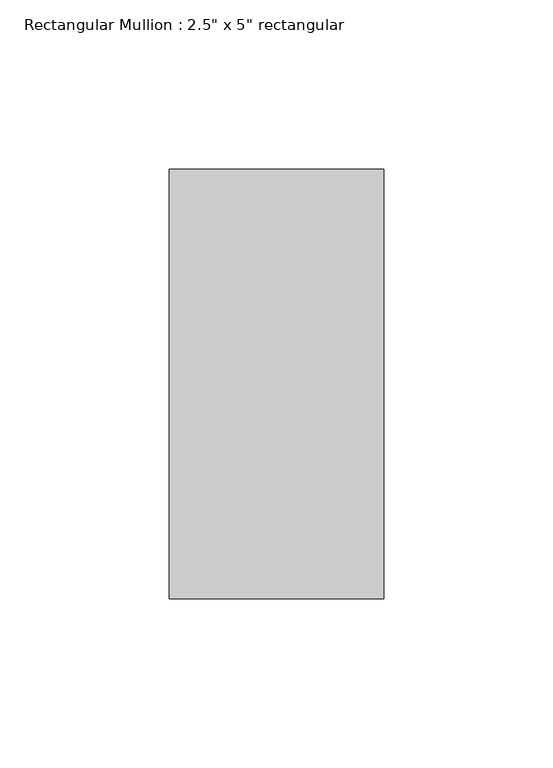
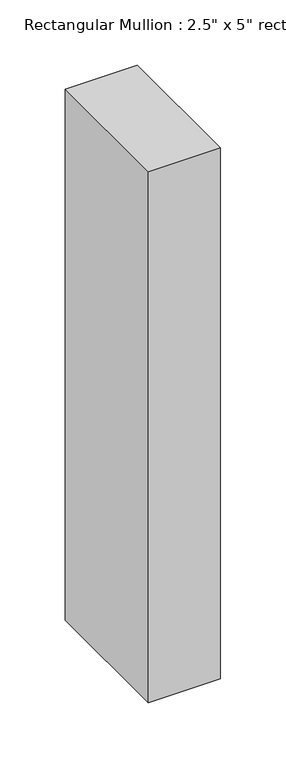
"""IFC4 building model written with IfcOpenShell, lengths in millimetres: member geometry."""

from ifc_helpers import new_model, si_unit, frame, origin, place, context, project, spatial, polyline, outline, extrude, source, transform, mapped, element, save


def member_2ebf4a73(model_context):
    return source(origin(), model_context, "Body", "SweptSolid", [
        extrude(outline(polyline([(0.0, 63.5), (0.0, -63.5), (-63.5, -63.5), (-63.5, 63.5), (0.0, 63.5)])), frame((0.0, 0.0, -495.3), z_axis=(0.0, 0.0, 1.0), x_axis=(1.0, 0.0, 0.0)), (0.0, 0.0, 1.0), 495.3),
    ])


if __name__ == "__main__":
    model = new_model("IFC4")
    model_context = context("Model", 3, world=origin())
    ifc_project = project(units=[si_unit("LENGTHUNIT", "METRE", prefix="MILLI")], contexts=[model_context])
    site = spatial("IfcSite", under=ifc_project)
    building = spatial("IfcBuilding", under=site)
    placement = place(None, origin())
    member_shape = member_2ebf4a73(model_context)
    element("IfcMember", 1, ObjectType="Rectangular Mullion : 2.5\" x 5\" rectangular", at=placement, inside=building, context=model_context, shape_type="MappedRepresentation", body=[
        mapped(member_shape, transform((0.0, 0.0, 0.0), x_axis=(1.0, 0.0, 0.0), y_axis=(0.0, 1.0, 0.0), z_axis=(0.0, 0.0, 1.0))),
    ])
    save(model, "model.ifc")

# Revit data of these elements
# Type "Rectangular Mullion : 2.5\" x 5\" rectangular"
#   built-in parameter 1007304 = 0.416667 (stored number, unit not read)
#   built-in parameter 1007301 = 0.104167 (stored number, unit not read)
#   built-in parameter 1007300 = 0.104167 (stored number, unit not read)
# Element 1 (IfcMember, "Rectangular Mullion : 2.5\" x 5\" rectangular")
#   Materials on its faces: "door colour"
# Materials
#   "door colour": class "Generic", colour RGB 120 120 120, transparency 0, Cost = 0
